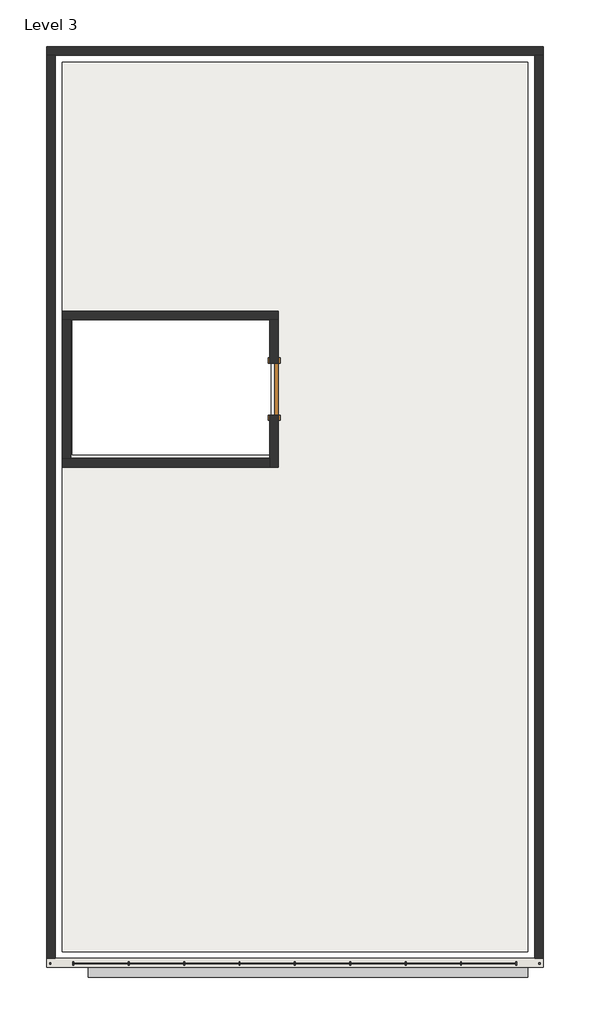
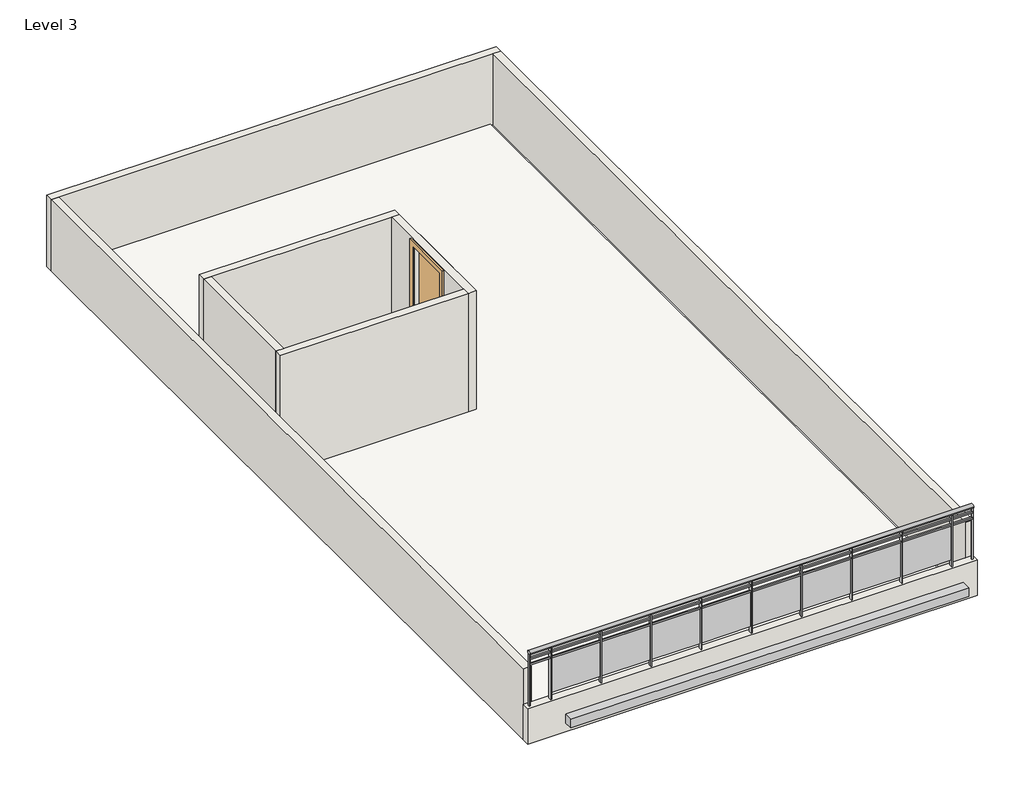
# One storey: 8 walls, 1 door, 1 proxy, 1 railing, 1 slab.
"""IFC4 building model written with IfcOpenShell, lengths in millimetres."""

from ifc_helpers import new_model, si_unit, point, frame, origin, place, context, project, spatial, polyline, ellipse_curve, trimmed, outline, extrude, faceted_brep, transform, mapped, element, save
from ifc_brep_helpers import plane_surface, extruded_surface, advanced_brep
from components import generic_models_10_generic_models_10_b1b5e2eb, door_1fe7f57d

model = new_model("IFC4")

# Units and contexts
model_context = context("Model", 3, world=origin())
ifc_project = project(units=[si_unit("LENGTHUNIT", "METRE", prefix="MILLI")], contexts=[model_context])

# Site, building, storey
site = spatial("IfcSite", under=ifc_project)
building = spatial("IfcBuilding", under=site)
storey = spatial("IfcBuildingStorey", under=building, Name="Level 3", Elevation=6400.8)

# Proxy
placement = place(None, origin())
generic_models_10_generic_models_10_shape = generic_models_10_generic_models_10_b1b5e2eb(model_context)
element("IfcBuildingElementProxy", 1, Name="Generic Models 10 : Generic Models 10", ObjectType="Generic Models 10 : Generic Models 10", at=placement, inside=storey, context=model_context, shape_type="MappedRepresentation", body=[
    mapped(generic_models_10_generic_models_10_shape, transform((0.0, 0.0, 0.0), x_axis=(1.0, 0.0, 0.0), y_axis=(0.0, 1.0, 0.0), z_axis=(0.0, 0.0, 1.0))),
])

# Door
door_shape = door_1fe7f57d(model_context)
element("IfcDoor", 2, ObjectType="Single-Flush : 30\" x 80\"", at=placement, inside=storey, context=model_context, shape_type="MappedRepresentation", body=[
    mapped(door_shape, transform((-6358.0482439, 2761.0172538, 6400.8), x_axis=(0.0, -1.0, 0.0), y_axis=(1.0, 0.0, 0.0), z_axis=(0.0, 0.0, 1.0))),
])

# Railing
element("IfcRailing", 3, ObjectType="Glass Panel - Bottom Fill", at=placement, inside=storey, context=model_context, shape_type="SolidModel", body=[
    advanced_brep(
    [(-9647.3482439, -5633.6827462, 7924.8), (-9647.3482439, -5709.8827462, 7924.8), (-2459.1482439, -5633.6827462, 7924.8), (-2459.1482439, -5709.8827462, 7924.8)],
    [
        (0, 1, ellipse_curve(frame((-9647.3482439, -5671.7827462, 7924.8), z_axis=(-1.0, 0.0, 0.0), x_axis=(0.0, -1.0, 0.0)), 38.1, 28.575)),
        (1, 0, ellipse_curve(frame((-9647.3482439, -5671.7827462, 7924.8), z_axis=(-1.0, 0.0, 0.0), x_axis=(0.0, -1.0, 0.0)), 38.1, 28.575)),
        (2, 3, ellipse_curve(frame((-2459.1482439, -5671.7827462, 7924.8), z_axis=(1.0, 0.0, 0.0), x_axis=(0.0, -1.0, 0.0)), 38.1, 28.575)),
        (3, 2, ellipse_curve(frame((-2459.1482439, -5671.7827462, 7924.8), z_axis=(1.0, 0.0, 0.0), x_axis=(0.0, -1.0, 0.0)), 38.1, 28.575)),
        (0, 2),
        (3, 1),
    ],
    [
        plane_surface(frame((-9647.3482439, -5671.7827462, 7924.8), z_axis=(-1.0, 0.0, 0.0), x_axis=(0.0, 1.0, 0.0))),
        plane_surface(frame((-2459.1482439, -5671.7827462, 7924.8), z_axis=(1.0, 0.0, 0.0), x_axis=(0.0, 1.0, 0.0))),
        extruded_surface(trimmed(ellipse_curve(frame((-2459.1482439, -5671.7827462, 7924.8), z_axis=(-1.0, 0.0, 0.0), x_axis=(0.0, -1.0, 0.0)), 38.1, 28.575), [point((-2459.1482439, -5633.6827462, 7924.8))], [point((-2459.1482439, -5709.8827462, 7924.8))], True, "CARTESIAN"), (-7188.2, 0.0, 0.0), 7188.2),
        extruded_surface(trimmed(ellipse_curve(frame((-2459.1482439, -5671.7827462, 7924.8), z_axis=(-1.0, 0.0, 0.0), x_axis=(0.0, -1.0, 0.0)), 38.1, 28.575), [point((-2459.1482439, -5709.8827462, 7924.8))], [point((-2459.1482439, -5633.6827462, 7924.8))], True, "CARTESIAN"), (-7188.2, 0.0, 0.0), 7188.2),
    ],
    [
        (0, [[1, 2]]),
        (1, [[3, 4]]),
        (2, [[-1, 5, -4, 6]]),
        (3, [[-2, -6, -3, -5]]),
    ],
),
    extrude(outline(polyline([(-9647.3482439, -5684.4827462), (-9647.3482439, -5659.0827462), (-2459.1482439, -5659.0827462), (-2459.1482439, -5684.4827462), (-9647.3482439, -5684.4827462)])), frame((0.0, 0.0, 7810.5), z_axis=(0.0, 0.0, 1.0), x_axis=(1.0, 0.0, 0.0)), (0.0, 0.0, 1.0), 25.4),
    extrude(outline(polyline([(-9647.3482439, -5684.4827462), (-9647.3482439, -5659.0827462), (-2459.1482439, -5659.0827462), (-2459.1482439, -5684.4827462), (-9647.3482439, -5684.4827462)])), frame((0.0, 0.0, 7708.9), z_axis=(0.0, 0.0, 1.0), x_axis=(1.0, 0.0, 0.0)), (0.0, 0.0, 1.0), 25.4),
    extrude(outline(polyline([(-2808.3982439, -5697.1827462), (-2808.3982439, -5646.3827462), (-2795.6982439, -5646.3827462), (-2795.6982439, -5697.1827462), (-2808.3982439, -5697.1827462)])), frame((0.0, 0.0, 7010.4), z_axis=(0.0, 0.0, 1.0), x_axis=(1.0, 0.0, 0.0)), (0.0, 0.0, 1.0), 885.825),
    extrude(outline(polyline([(-3614.8482439, -5665.2475892), (-2802.0482439, -5665.2475892), (-2802.0482439, -5671.5975892), (-3614.8482439, -5671.5975892), (-3614.8482439, -5665.2475892)])), frame((0.0, 0.0, 7112.0), z_axis=(0.0, 0.0, 1.0), x_axis=(1.0, 0.0, 0.0)), (0.0, 0.0, 1.0), 596.9),
    extrude(outline(polyline([(-3621.1982439, -5697.1827462), (-3621.1982439, -5646.3827462), (-3608.4982439, -5646.3827462), (-3608.4982439, -5697.1827462), (-3621.1982439, -5697.1827462)])), frame((0.0, 0.0, 7010.4), z_axis=(0.0, 0.0, 1.0), x_axis=(1.0, 0.0, 0.0)), (0.0, 0.0, 1.0), 885.825),
    extrude(outline(polyline([(-4427.6482439, -5665.2475892), (-3614.8482439, -5665.2475892), (-3614.8482439, -5671.5975892), (-4427.6482439, -5671.5975892), (-4427.6482439, -5665.2475892)])), frame((0.0, 0.0, 7112.0), z_axis=(0.0, 0.0, 1.0), x_axis=(1.0, 0.0, 0.0)), (0.0, 0.0, 1.0), 596.9),
    extrude(outline(polyline([(-4433.9982439, -5697.1827462), (-4433.9982439, -5646.3827462), (-4421.2982439, -5646.3827462), (-4421.2982439, -5697.1827462), (-4433.9982439, -5697.1827462)])), frame((0.0, 0.0, 7010.4), z_axis=(0.0, 0.0, 1.0), x_axis=(1.0, 0.0, 0.0)), (0.0, 0.0, 1.0), 885.825),
    extrude(outline(polyline([(-5240.4482439, -5665.2475892), (-4427.6482439, -5665.2475892), (-4427.6482439, -5671.5975892), (-5240.4482439, -5671.5975892), (-5240.4482439, -5665.2475892)])), frame((0.0, 0.0, 7112.0), z_axis=(0.0, 0.0, 1.0), x_axis=(1.0, 0.0, 0.0)), (0.0, 0.0, 1.0), 596.9),
    extrude(outline(polyline([(-5246.7982439, -5697.1827462), (-5246.7982439, -5646.3827462), (-5234.0982439, -5646.3827462), (-5234.0982439, -5697.1827462), (-5246.7982439, -5697.1827462)])), frame((0.0, 0.0, 7010.4), z_axis=(0.0, 0.0, 1.0), x_axis=(1.0, 0.0, 0.0)), (0.0, 0.0, 1.0), 885.825),
    extrude(outline(polyline([(-6053.2482439, -5665.2475892), (-5240.4482439, -5665.2475892), (-5240.4482439, -5671.5975892), (-6053.2482439, -5671.5975892), (-6053.2482439, -5665.2475892)])), frame((0.0, 0.0, 7112.0), z_axis=(0.0, 0.0, 1.0), x_axis=(1.0, 0.0, 0.0)), (0.0, 0.0, 1.0), 596.9),
    extrude(outline(polyline([(-6059.5982439, -5697.1827462), (-6059.5982439, -5646.3827462), (-6046.8982439, -5646.3827462), (-6046.8982439, -5697.1827462), (-6059.5982439, -5697.1827462)])), frame((0.0, 0.0, 7010.4), z_axis=(0.0, 0.0, 1.0), x_axis=(1.0, 0.0, 0.0)), (0.0, 0.0, 1.0), 885.825),
    extrude(outline(polyline([(-6866.0482439, -5665.2475892), (-6053.2482439, -5665.2475892), (-6053.2482439, -5671.5975892), (-6866.0482439, -5671.5975892), (-6866.0482439, -5665.2475892)])), frame((0.0, 0.0, 7112.0), z_axis=(0.0, 0.0, 1.0), x_axis=(1.0, 0.0, 0.0)), (0.0, 0.0, 1.0), 596.9),
    extrude(outline(polyline([(-6872.3982439, -5697.1827462), (-6872.3982439, -5646.3827462), (-6859.6982439, -5646.3827462), (-6859.6982439, -5697.1827462), (-6872.3982439, -5697.1827462)])), frame((0.0, 0.0, 7010.4), z_axis=(0.0, 0.0, 1.0), x_axis=(1.0, 0.0, 0.0)), (0.0, 0.0, 1.0), 885.825),
    extrude(outline(polyline([(-7678.8482439, -5665.2475892), (-6866.0482439, -5665.2475892), (-6866.0482439, -5671.5975892), (-7678.8482439, -5671.5975892), (-7678.8482439, -5665.2475892)])), frame((0.0, 0.0, 7112.0), z_axis=(0.0, 0.0, 1.0), x_axis=(1.0, 0.0, 0.0)), (0.0, 0.0, 1.0), 596.9),
    extrude(outline(polyline([(-7685.1982439, -5697.1827462), (-7685.1982439, -5646.3827462), (-7672.4982439, -5646.3827462), (-7672.4982439, -5697.1827462), (-7685.1982439, -5697.1827462)])), frame((0.0, 0.0, 7010.4), z_axis=(0.0, 0.0, 1.0), x_axis=(1.0, 0.0, 0.0)), (0.0, 0.0, 1.0), 885.825),
    extrude(outline(polyline([(-8491.6482439, -5665.2475892), (-7678.8482439, -5665.2475892), (-7678.8482439, -5671.5975892), (-8491.6482439, -5671.5975892), (-8491.6482439, -5665.2475892)])), frame((0.0, 0.0, 7112.0), z_axis=(0.0, 0.0, 1.0), x_axis=(1.0, 0.0, 0.0)), (0.0, 0.0, 1.0), 596.9),
    extrude(outline(polyline([(-8497.9982439, -5697.1827462), (-8497.9982439, -5646.3827462), (-8485.2982439, -5646.3827462), (-8485.2982439, -5697.1827462), (-8497.9982439, -5697.1827462)])), frame((0.0, 0.0, 7010.4), z_axis=(0.0, 0.0, 1.0), x_axis=(1.0, 0.0, 0.0)), (0.0, 0.0, 1.0), 885.825),
    extrude(outline(polyline([(-9304.4482439, -5665.2475892), (-8491.6482439, -5665.2475892), (-8491.6482439, -5671.5975892), (-9304.4482439, -5671.5975892), (-9304.4482439, -5665.2475892)])), frame((0.0, 0.0, 7112.0), z_axis=(0.0, 0.0, 1.0), x_axis=(1.0, 0.0, 0.0)), (0.0, 0.0, 1.0), 596.9),
    extrude(outline(polyline([(-9310.7982439, -5697.1827462), (-9310.7982439, -5646.3827462), (-9298.0982439, -5646.3827462), (-9298.0982439, -5697.1827462), (-9310.7982439, -5697.1827462)])), frame((0.0, 0.0, 7010.4), z_axis=(0.0, 0.0, 1.0), x_axis=(1.0, 0.0, 0.0)), (0.0, 0.0, 1.0), 885.825),
    extrude(outline(polyline([(-2471.8482439, -5681.3077462), (-2471.8482439, -5662.2577462), (-2452.7982439, -5662.2577462), (-2452.7982439, -5681.3077462), (-2471.8482439, -5681.3077462)])), frame((0.0, 0.0, 7010.4), z_axis=(0.0, 0.0, 1.0), x_axis=(1.0, 0.0, 0.0)), (0.0, 0.0, 1.0), 885.825),
    extrude(outline(polyline([(-9653.6982439, -5681.3077462), (-9653.6982439, -5662.2577462), (-9634.6482439, -5662.2577462), (-9634.6482439, -5681.3077462), (-9653.6982439, -5681.3077462)])), frame((0.0, 0.0, 7010.4), z_axis=(0.0, 0.0, 1.0), x_axis=(1.0, 0.0, 0.0)), (0.0, 0.0, 1.0), 885.825),
])

# Slab
element("IfcSlab", 4, ObjectType="carpet finishing 6\"", at=placement, inside=storey, context=model_context, shape_type="SweptSolid", body=[
    extrude(outline(polyline([(-2636.9482439, 7563.2047538), (-2636.9482439, -5493.9827462), (-9471.1357439, -5493.9827462), (-9471.1357439, 7563.2047538), (-2636.9482439, 7563.2047538)]), holes=[polyline([(-9317.1482439, 3777.0172538), (-9317.1482439, 1795.8172538), (-6410.3576348, 1795.8172538), (-6410.3576348, 3777.0172538), (-9317.1482439, 3777.0172538)])]), frame((0.0, 0.0, 6350.0), z_axis=(0.0, 0.0, 1.0), x_axis=(1.0, 0.0, 0.0)), (0.0, 0.0, 1.0), 152.4),
])

# Walls
element("IfcWall", 5, ObjectType="INNER WALL 5\"", at=placement, inside=storey, context=model_context, shape_type="Brep", body=[
    faceted_brep([(-9469.6364384, 3777.0172538, 6400.8), (-9342.6364077, 3777.0172538, 6400.8), (-6421.5482439, 3777.0172538, 6400.8), (-6294.5482439, 3777.0172538, 6400.8), (-6294.5482439, 3777.0172538, 8534.4), (-6421.5482439, 3777.0172538, 8534.4), (-9342.6364077, 3777.0172538, 8534.4), (-9469.6364384, 3777.0172538, 8534.4), (-9469.5482439, 3904.0172538, 6400.8), (-9469.5482439, 3904.0172538, 8534.4), (-6294.5482439, 3904.0172538, 8534.4), (-6294.5482439, 3904.0172538, 6400.8)], [[[0, 1, 2, 3, 4, 5, 6, 7]], [[8, 9, 10, 11]], [[3, 2, 1, 0, 8, 11]], [[7, 6, 5, 4, 10, 9]], [[4, 3, 11, 10]], [[0, 7, 9, 8]]]),
])
element("IfcWall", 6, ObjectType="INNER WALL 5\"", at=placement, inside=storey, context=model_context, shape_type="Brep", body=[
    faceted_brep([(-6421.5482439, 2380.0172538, 8432.8), (-6421.5482439, 2380.0172538, 6400.8), (-6421.5482439, 1745.0172538, 6400.8), (-6421.5482439, 1618.0172538, 6400.8), (-6421.5482439, 1618.0172538, 8534.4), (-6421.5482439, 1745.0172538, 8534.4), (-6421.5482439, 3777.0172538, 8534.4), (-6421.5482439, 3777.0172538, 6400.8), (-6421.5482439, 3142.0172538, 6400.8), (-6421.5482439, 3142.0172538, 8432.8), (-6294.5482439, 1618.0172538, 6400.8), (-6294.5482439, 2380.0172538, 6400.8), (-6294.5482439, 2380.0172538, 8432.8), (-6294.5482439, 3142.0172538, 8432.8), (-6294.5482439, 3142.0172538, 6400.8), (-6294.5482439, 3777.0172538, 6400.8), (-6294.5482439, 3777.0172538, 8534.4), (-6294.5482439, 1618.0172538, 8534.4)], [[[0, 1, 2, 3, 4, 5, 6, 7, 8, 9]], [[10, 11, 12, 13, 14, 15, 16, 17]], [[8, 7, 15, 14]], [[3, 2, 1, 11, 10]], [[6, 5, 4, 17, 16]], [[7, 6, 16, 15]], [[4, 3, 10, 17]], [[12, 11, 1, 0]], [[13, 12, 0, 9]], [[14, 13, 9, 8]]]),
])
element("IfcWall", 7, ObjectType="INNER WALL 5\"", at=placement, inside=storey, context=model_context, shape_type="Brep", body=[
    faceted_brep([(-6421.5482439, 1745.0172538, 6400.8), (-9344.0475188, 1745.0172538, 6400.8), (-9471.0475495, 1745.0172538, 6400.8), (-9471.0475495, 1745.0172538, 8534.4), (-9344.0475188, 1745.0172538, 8534.4), (-6421.5482439, 1745.0172538, 8534.4), (-6421.5482439, 1618.0172538, 6400.8), (-6421.5482439, 1618.0172538, 8534.4), (-9471.1357439, 1618.0172538, 8534.4), (-9471.1357439, 1618.0172538, 6400.8)], [[[0, 1, 2, 3, 4, 5]], [[6, 7, 8, 9]], [[2, 1, 0, 6, 9]], [[5, 4, 3, 8, 7]], [[0, 5, 7, 6]], [[3, 2, 9, 8]]]),
])
element("IfcWall", 8, ObjectType="INNER WALL 5\"", at=placement, inside=storey, context=model_context, shape_type="SweptSolid", body=[
    extrude(outline(polyline([(-9342.6364077, 3777.0172538), (-9344.0475188, 1745.0172538), (-9471.0475495, 1745.0172538), (-9469.6364384, 3777.0172538), (-9342.6364077, 3777.0172538)])), frame((0.0, 0.0, 6400.8), z_axis=(0.0, 0.0, 1.0), x_axis=(1.0, 0.0, 0.0)), (0.0, 0.0, 1.0), 2133.6),
])
element("IfcWall", 9, ObjectType="INNER WALL 5\"", at=placement, inside=storey, context=model_context, shape_type="Brep", body=[
    faceted_brep([(-9698.1482439, 7663.2172538, 6400.8), (-9571.1482439, 7663.2172538, 6400.8), (-2533.7607439, 7663.2172538, 6400.8), (-2406.7607439, 7663.2172538, 6400.8), (-2406.7607439, 7663.2172538, 7620.0), (-2533.7607439, 7663.2172538, 7620.0), (-9571.1482439, 7663.2172538, 7620.0), (-9698.1482439, 7663.2172538, 7620.0), (-9698.1482439, 7790.2172538, 6400.8), (-9698.1482439, 7790.2172538, 7620.0), (-2406.7607439, 7790.2172538, 7620.0), (-2406.7607439, 7790.2172538, 6400.8)], [[[0, 1, 2, 3, 4, 5, 6, 7]], [[8, 9, 10, 11]], [[3, 2, 1, 0, 8, 11]], [[7, 6, 5, 4, 10, 9]], [[4, 3, 11, 10]], [[0, 7, 9, 8]]]),
])
element("IfcWall", 10, ObjectType="INNER WALL 5\"", at=placement, inside=storey, context=model_context, shape_type="Brep", body=[
    faceted_brep([(-2533.7607439, 7663.2172538, 6400.8), (-2533.7607439, -5595.5827462, 6400.8), (-2533.7607439, -5595.5827462, 7620.0), (-2533.7607439, 7663.2172538, 7620.0), (-2406.7607439, 7663.2172538, 6400.8), (-2406.7607439, 7663.2172538, 7620.0), (-2406.7607439, -5595.5827462, 7620.0), (-2406.7607439, -5595.5827462, 7010.4), (-2406.7607439, -5595.5827462, 6400.8)], [[[0, 1, 2, 3]], [[4, 5, 6, 7, 8]], [[1, 0, 4, 8]], [[3, 2, 6, 5]], [[0, 3, 5, 4]], [[2, 1, 8, 7, 6]]]),
])
element("IfcWall", 11, ObjectType="INNER WALL 5\"", at=placement, inside=storey, context=model_context, shape_type="Brep", body=[
    faceted_brep([(-2406.7607439, -5595.5827462, 6400.8), (-2533.7607439, -5595.5827462, 6400.8), (-9571.1482439, -5595.5827462, 6400.8), (-9698.1482439, -5595.5827462, 6400.8), (-9698.1482439, -5595.5827462, 7010.4), (-2406.7607439, -5595.5827462, 7010.4), (-2406.7607439, -5722.5827462, 6400.8), (-2406.7607439, -5722.5827462, 7010.4), (-9698.1482439, -5722.5827462, 7010.4), (-9698.1482439, -5722.5827462, 6400.8)], [[[0, 1, 2, 3, 4, 5]], [[6, 7, 8, 9]], [[3, 2, 1, 0, 6, 9]], [[5, 4, 8, 7]], [[4, 3, 9, 8]], [[0, 5, 7, 6]]]),
])
element("IfcWall", 12, ObjectType="INNER WALL 5\"", at=placement, inside=storey, context=model_context, shape_type="Brep", body=[
    faceted_brep([(-9571.1482439, -5595.5827462, 6400.8), (-9571.1482439, 7663.2172538, 6400.8), (-9571.1482439, 7663.2172538, 7620.0), (-9571.1482439, -5595.5827462, 7620.0), (-9698.1482439, -5595.5827462, 6400.8), (-9698.1482439, -5595.5827462, 7010.4), (-9698.1482439, -5595.5827462, 7620.0), (-9698.1482439, 7663.2172538, 7620.0), (-9698.1482439, 7663.2172538, 6400.8)], [[[0, 1, 2, 3]], [[4, 5, 6, 7, 8]], [[1, 0, 4, 8]], [[3, 2, 7, 6]], [[0, 3, 6, 5, 4]], [[2, 1, 8, 7]]]),
])

save(model, "model.ifc")

# Revit data of these elements
# Type "Single-Flush : 30\" x 80\""
#   Type Mark = "5"
#   Construction Type Id = "MDOOR"
#   Assembly Code = "C1020"
#   Analytic Construction = "Metal"
#   Thickness = 0' - 2"
#   Heat Transfer Coefficient (U) = 0.651978 BTU/(h·ft²·°F)
#   Height = 6' - 8"
#   Trim Projection Ext = 0' - 1"
#   Trim Projection Int = 0' - 1"
#   Trim Width = 0' - 3"
#   Width = 2' - 6"
#   Define Thermal Properties by = 1
#   Define Thermal Properties by = 1
#   Door Material = Door - Panel
#   Frame Material = Door - Frame
#   Visual Light Transmittance = 0
#   Solar Heat Gain Coefficient = 0
#   Function = (empty or 0)
#   Wall Closure = (empty or 0)
# Type "Glass Panel - Bottom Fill"
#   Assembly Code = "C2010400"
#   built-in parameter 1008612 = 0.0416667 (stored number, unit not read)
#   built-in parameter 1008611 = 0.0416667 (stored number, unit not read)
#   built-in parameter 1008609 = 0.333333 (stored number, unit not read)
#   built-in parameter 1008604 = 0.166667 (stored number, unit not read)
#   built-in parameter 1008603 = 0.166667 (stored number, unit not read)
#   Railing Height = 3' - 0"
#   built-in parameter 1008630 = 2
#   built-in parameter 1008610 = 2
#   built-in parameter 1008618 = Baluster - Square : 3/4"
# Type "carpet finishing 6\""
#   Assembly Code = "B1010"
#   Function = 0
#   Layers, outside or top first: 0' - 6" "CARPET FINISHING" (function 1)
# Type "INNER WALL 5\""
#   Assembly Code = "B2010"
# Element 1 (IfcBuildingElementProxy, "Generic Models 10 : Generic Models 10")
#   Phase Created = New Construction
#   Materials on its faces: "GLASS MATERIAL"
# Element 2 (IfcDoor, "Single-Flush : 30\" x 80\"")
#   Phase Created = New Construction
#   Materials on its faces: "Door - Frame", "Door - Panel"
# Element 3 (IfcRailing, "Glass Panel - Bottom Fill")
#   built-in parameter 1008621 = 2 (stored number, unit not read)
#   Phase Created = New Construction
#   Materials on its faces: "Glass", "BLACK"
# Element 4 (IfcSlab, "carpet finishing 6\"")
#   Height Offset From Level = 0' - 4"
#   Phase Created = New Construction
#   Materials on its faces: "CARPET FINISHING"
# Elements 5, 6, 7, 8 (IfcWall, "INNER WALL 5\"")
#   Top Offset = 0' - 0"
#   Base Offset = 0' - 0"
#   Unconnected Height = 7' - 0"
#   wall height = 7' - 0"
#   Phase Created = New Construction
#   Base Constraint = Level 3
# Elements 9, 10, 12 (IfcWall, "INNER WALL 5\"")
#   Top Offset = 0' - 0"
#   Base Offset = 0' - 0"
#   Unconnected Height = 4' - 0"
#   wall height = 4' - 0"
#   Phase Created = New Construction
#   Base Constraint = Level 3
# Element 11 (IfcWall, "INNER WALL 5\"")
#   Top Offset = 0' - 0"
#   Base Offset = 0' - 0"
#   Unconnected Height = 2' - 0"
#   wall height = 2' - 0"
#   Phase Created = New Construction
#   Base Constraint = Level 3
# Materials
#   "Door - Panel": class "Wood", colour RGB 210 159 95, transparency 0, Cost = 0
#   "Door - Frame": colour RGB 118 70 51, transparency 0, Cost = 0
#   "CARPET FINISHING": class "Generic", colour RGB 120 120 120, transparency 0, Cost = 0
#   "GLASS MATERIAL": class "Generic", colour RGB 120 120 120, transparency 0, Cost = 0
#   "Glass": class "Glass", colour RGB 0 128 192, transparency 0.75, Description = "Soda Lime Glass", Cost = 0
#   "BLACK": class "Generic", colour RGB 120 120 120, transparency 0, Cost = 0
